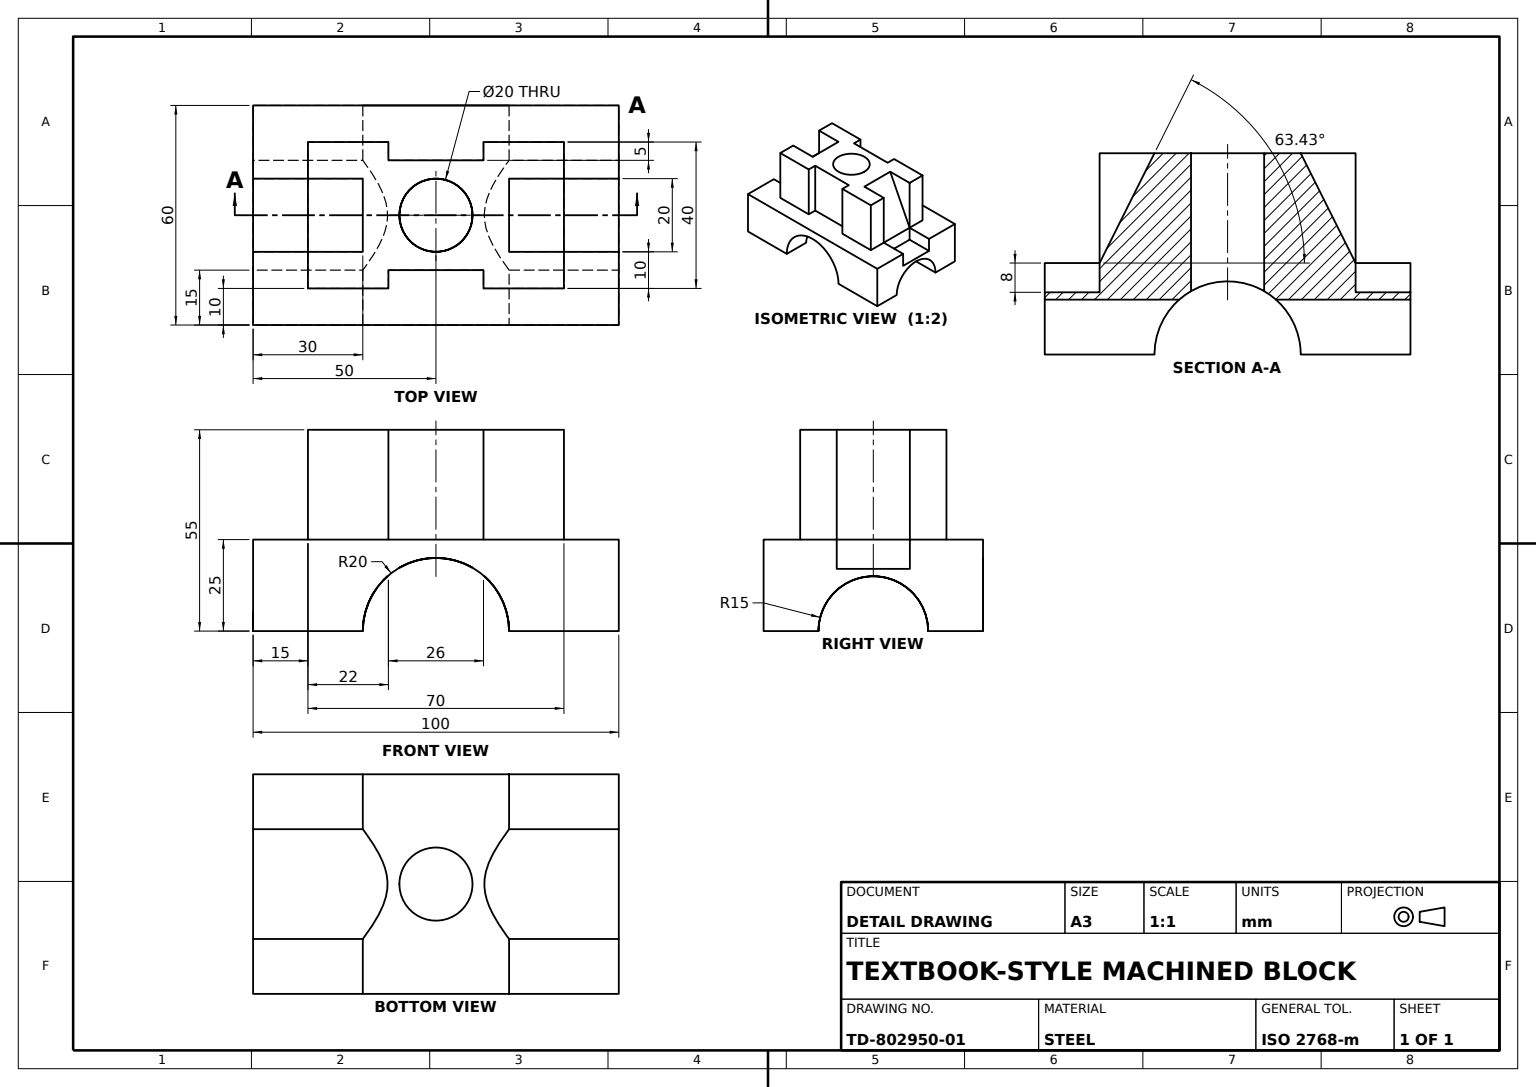
SolidWorks part; units mm, degrees
material "Plain Carbon Steel"
ref_plane "Front Plane" through (0, 0, 0) normal (0, 0, 1) x (1, 0, 0)
ref_plane "Top Plane" through (0, 0, 0) normal (0, 1, 0) x (1, 0, 0)
ref_plane "Right Plane" through (0, 0, 0) normal (1, 0, 0) x (0, 0, -1)
sketch "Base Block Profile" plane through (0, 0, 0) normal (1, 0, 0) x (0, 0, -1)
  line L1 (-50, 12.5) -> (50, 12.5)
  line L2 (-50, 12.5) -> (-50, -12.5)
  line L3 (-50, -12.5) -> (50, -12.5)
  line L4 (50, 12.5) -> (50, -12.5)
  line L5 (-50, 12.5) -> (50, -12.5) construction
  line L6 (-50, -12.5) -> (50, 12.5) construction
  point P0 (0, 0)
  dimension "D1" = 25
  dimension "D2" = 100
extrude "Base Block" add sketch "Base Block Profile" along normal mid plane 60
sketch "End Arch Profile" plane through (0, 0, 50) normal (0, 0, 1) x (1, 0, 0)
  line L0 (30, -12.5) -> (-30, -12.5) construction
  arc A0 (-15, -12.5) -> (15, -12.5) centre (0, -12.5) cw
  line M3 (-30, -12.5) -> (30, -12.5)
  dimension "D1" = 15
extrude "End Arch Cut" cut sketch "End Arch Profile" against normal through all both and the other way through all contours A0 M3
sketch "Center Arch Profile" plane through (30, 0, 0) normal (1, 0, 0) x (0, 0, -1)
  line L0 (-50, -12.5) -> (50, -12.5) construction
  arc A0 (-20, -12.5) -> (20, -12.5) centre (0, -12.5) cw
  line M5 (-50, -12.5) -> (50, -12.5)
  dimension "D1" = 20
extrude "Center Arch Cut" cut sketch "Center Arch Profile" against normal through all contours A0 M5
sketch "Upper Block Profile" plane through (0, 0, 0) normal (0, 0, 1) x (1, 0, 0)
  line L0 (30, 12.5) -> (-30, 12.5) construction
  line L1 (-20, 12.5) -> (20, 12.5)
  line L2 (-20, 12.5) -> (-20, 42.5)
  line L3 (-20, 42.5) -> (20, 42.5)
  line L4 (20, 12.5) -> (20, 42.5)
  point P6 (0, 42.5)
  dimension "D1" = 40
  dimension "D2" = 30
extrude "Upper Block" add sketch "Upper Block Profile" along normal mid plane 70
sketch "Side Slot Profile" plane through (0, 42.5, 0) normal (0, 1, 0) x (1, 0, 0)
  line L0 (20, -35) -> (20, 35) construction
  line L1 (20, 13) -> (15, 13)
  line L2 (20, 13) -> (20, -13)
  line L3 (20, -13) -> (15, -13)
  line L4 (15, 13) -> (15, -13)
  point P6 (20, 0)
  dimension "D1" = 26
  dimension "D2" = 5
extrude "Side Slot" cut sketch "Side Slot Profile" against normal up to surface (30 mm away) up to face at (0, 12.5, 0)
mirror "Side Slot Mirror" about plane through (0, 0, 0) normal (1, 0, 0) of "Side Slot"
sketch "Top Bore Profile" plane through (0, 42.5, 0) normal (0, 1, 0) x (1, 0, 0)
  circle A0 centre (0, 0) radius 10
  dimension "D1" = 20
extrude "Top Bore Ø20" cut sketch "Top Bore Profile" against normal through all
sketch "Base Notch Profile" plane through (0, 0, 50) normal (0, 0, 1) x (1, 0, 0)
  line L0 (30, 12.5) -> (-30, 12.5) construction
  line L1 (-10, 12.5) -> (10, 12.5)
  line L2 (-10, 12.5) -> (-10, 4.5)
  line L3 (-10, 4.5) -> (10, 4.5)
  line L4 (10, 12.5) -> (10, 4.5)
  point P6 (0, 4.5)
  dimension "D1" = 8
  dimension "D2" = 20
extrude "Base Notch" cut sketch "Base Notch Profile" against normal blind 15
sketch "Triangular Relief Profile" plane through (0, 0, 0) normal (1, 0, 0) x (0, 0, -1)
  line L0 (-35, 12.5) -> (-20, 42.5)
  line L1 (-35, 42.5) -> (-13, 42.5) construction
  line L2 (-20, 42.5) -> (-35, 42.5)
  line L3 (-35, 12.5) -> (-35, 42.5) construction
  line L4 (-35, 12.5) -> (-35, 42.5)
  dimension "D1" = 15
extrude "Triangular Relief Cut" cut sketch "Triangular Relief Profile" against normal mid plane 20
mirror "Notch and Relief Mirror" about plane through (0, 0, 0) normal (0, 0, 1) of "Base Notch", "Triangular Relief Cut"
